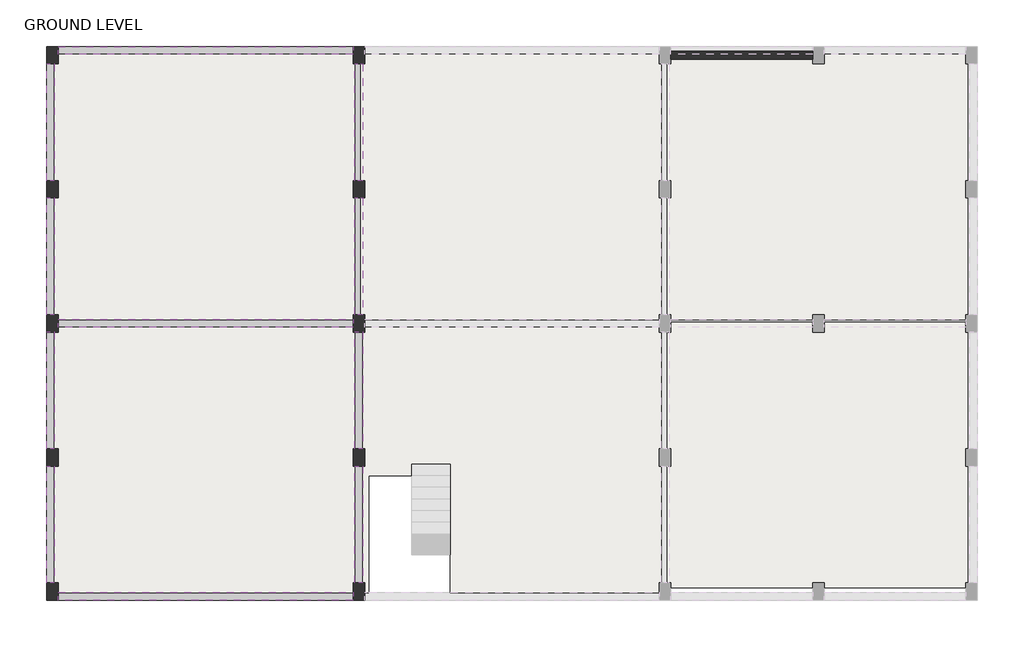
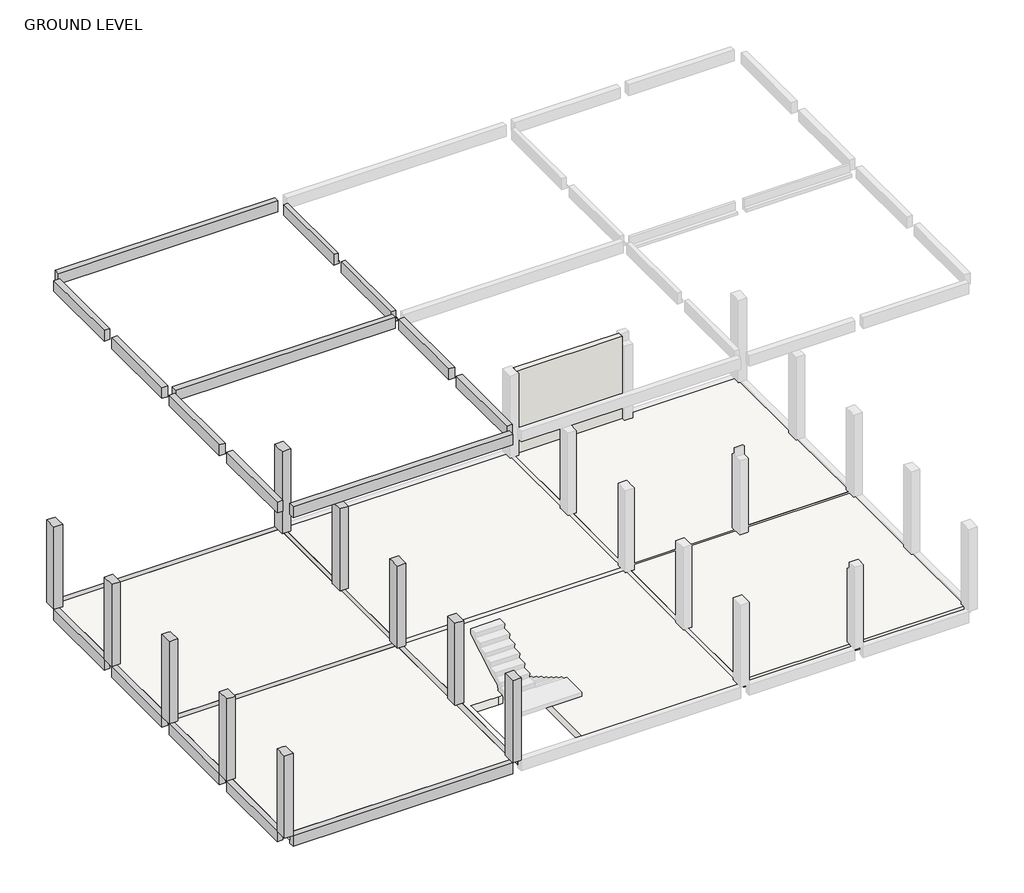
# One storey, part 1 of 2: 22 beams, 10 columns, 1 slab, 1 wall.
"""IFC4 building model written with IfcOpenShell, lengths in millimetres."""

from ifc_helpers import new_model, si_unit, frame, origin, place, context, project, spatial, polyline, outline, extrude, faceted_brep, element, save

model = new_model("IFC4")

# Units and contexts
model_context = context("Model", 3, world=origin())
ifc_project = project(units=[si_unit("LENGTHUNIT", "METRE", prefix="MILLI")], contexts=[model_context])

# Site, building, storey
site = spatial("IfcSite", under=ifc_project)
building = spatial("IfcBuilding", under=site)
storey = spatial("IfcBuildingStorey", under=building, Name="GROUND LEVEL", Elevation=0.0)

# Beams
placement = place(None, origin())
element("IfcBeam", 1, ObjectType="M_Concrete-Rectangular Beam : 200MMX400MM", at=placement, inside=storey, context=model_context, shape_type="Brep", body=[
    faceted_brep([(-3980.6874017, 15797.7008557, 0.0), (-3980.6874017, 15997.7008557, 0.0), (-11680.6874017, 15997.7008557, 0.0), (-11680.6874017, 15797.7008557, 0.0), (-3980.6874017, 15797.7008557, -400.0), (-3980.6874017, 15797.7008557, -300.0), (-11680.6874017, 15797.7008557, -300.0), (-11680.6874017, 15797.7008557, -400.0), (-3980.6874017, 15997.7008557, -400.0), (-11680.6874017, 15997.7008557, -400.0)], [[[0, 1, 2, 3]], [[4, 5, 0, 3, 6, 7]], [[8, 4, 7, 9]], [[1, 8, 9, 2]], [[2, 9, 7, 6, 3]], [[1, 0, 5, 4, 8]]]),
])
element("IfcBeam", 2, ObjectType="M_Concrete-Rectangular Beam : 200MMX400MM", at=placement, inside=storey, context=model_context, shape_type="Brep", body=[
    faceted_brep([(-11680.6874017, 1747.7008557, 0.0), (-11680.6874017, 1547.7008557, 0.0), (-3980.6874017, 1547.7008557, 0.0), (-3980.6874017, 1747.7008557, 0.0), (-11680.6874017, 1747.7008557, -400.0), (-11680.6874017, 1747.7008557, -300.0), (-3980.6874017, 1747.7008557, -300.0), (-3980.6874017, 1747.7008557, -400.0), (-11680.6874017, 1547.7008557, -400.0), (-3980.6874017, 1547.7008557, -400.0)], [[[0, 1, 2, 3]], [[4, 5, 0, 3, 6, 7]], [[8, 4, 7, 9]], [[1, 8, 9, 2]], [[1, 0, 5, 4, 8]], [[2, 9, 7, 6, 3]]]),
])
element("IfcBeam", 3, ObjectType="M_Concrete-Rectangular Beam : 200MMX400MM", at=placement, inside=storey, context=model_context, shape_type="Brep", body=[
    faceted_brep([(-3980.6874017, 8872.7008557, 0.0), (-11680.6874017, 8872.7008557, 0.0), (-11680.6874017, 8672.7008557, 0.0), (-3980.6874017, 8672.7008557, 0.0), (-11680.6874017, 8672.7008557, -300.0), (-11680.6874017, 8672.7008557, -400.0), (-3980.6874017, 8672.7008557, -400.0), (-3980.6874017, 8672.7008557, -300.0), (-11680.6874017, 8872.7008557, -400.0), (-3980.6874017, 8872.7008557, -400.0), (-3980.6874017, 8872.7008557, -300.0), (-11680.6874017, 8872.7008557, -300.0)], [[[0, 1, 2, 3]], [[3, 2, 4, 5, 6, 7]], [[6, 5, 8, 9]], [[1, 0, 10, 9, 8, 11]], [[8, 5, 4, 2, 1, 11]], [[0, 3, 7, 6, 9, 10]]]),
])
element("IfcBeam", 4, ObjectType="M_Concrete-Rectangular Beam : 200MMX400MM", at=placement, inside=storey, context=model_context, shape_type="Brep", body=[
    faceted_brep([(-11980.6874017, 12497.7008557, 0.0), (-11780.6874017, 12497.7008557, 0.0), (-11780.6874017, 15547.7008557, 0.0), (-11980.6874017, 15547.7008557, 0.0), (-11980.6874017, 12497.7008557, -400.0), (-11980.6874017, 15547.7008557, -400.0), (-11780.6874017, 12497.7008557, -400.0), (-11780.6874017, 15547.7008557, -400.0), (-11780.6874017, 12497.7008557, -300.0), (-11780.6874017, 15547.7008557, -300.0)], [[[0, 1, 2, 3]], [[4, 0, 3, 5]], [[6, 4, 5, 7]], [[1, 8, 6, 7, 9, 2]], [[2, 9, 7, 5, 3]], [[1, 0, 4, 6, 8]]]),
])
element("IfcBeam", 5, ObjectType="M_Concrete-Rectangular Beam : 200MMX400MM", at=placement, inside=storey, context=model_context, shape_type="Brep", body=[
    faceted_brep([(-11980.6874017, 8997.7008557, 0.0), (-11780.6874017, 8997.7008557, 0.0), (-11780.6874017, 12047.7008557, 0.0), (-11980.6874017, 12047.7008557, 0.0), (-11980.6874017, 8997.7008557, -400.0), (-11980.6874017, 12047.7008557, -400.0), (-11780.6874017, 8997.7008557, -400.0), (-11780.6874017, 12047.7008557, -400.0), (-11780.6874017, 8997.7008557, -300.0), (-11780.6874017, 12047.7008557, -300.0)], [[[0, 1, 2, 3]], [[4, 0, 3, 5]], [[6, 4, 5, 7]], [[1, 8, 6, 7, 9, 2]], [[1, 0, 4, 6, 8]], [[2, 9, 7, 5, 3]]]),
])
element("IfcBeam", 6, ObjectType="M_Concrete-Rectangular Beam : 200MMX400MM", at=placement, inside=storey, context=model_context, shape_type="Brep", body=[
    faceted_brep([(-11980.6874017, 5497.7008557, 0.0), (-11780.6874017, 5497.7008557, 0.0), (-11780.6874017, 8547.7008557, 0.0), (-11980.6874017, 8547.7008557, 0.0), (-11980.6874017, 5497.7008557, -400.0), (-11980.6874017, 8547.7008557, -400.0), (-11780.6874017, 5497.7008557, -400.0), (-11780.6874017, 8547.7008557, -400.0), (-11780.6874017, 5497.7008557, -300.0), (-11780.6874017, 8547.7008557, -300.0)], [[[0, 1, 2, 3]], [[4, 0, 3, 5]], [[6, 4, 5, 7]], [[1, 8, 6, 7, 9, 2]], [[2, 9, 7, 5, 3]], [[1, 0, 4, 6, 8]]]),
])
element("IfcBeam", 7, ObjectType="M_Concrete-Rectangular Beam : 200MMX400MM", at=placement, inside=storey, context=model_context, shape_type="Brep", body=[
    faceted_brep([(-11980.6874017, 1997.7008557, 0.0), (-11780.6874017, 1997.7008557, 0.0), (-11780.6874017, 5047.7008557, 0.0), (-11980.6874017, 5047.7008557, 0.0), (-11980.6874017, 1997.7008557, -400.0), (-11980.6874017, 5047.7008557, -400.0), (-11780.6874017, 1997.7008557, -400.0), (-11780.6874017, 5047.7008557, -400.0), (-11780.6874017, 1997.7008557, -300.0), (-11780.6874017, 5047.7008557, -300.0)], [[[0, 1, 2, 3]], [[4, 0, 3, 5]], [[6, 4, 5, 7]], [[1, 8, 6, 7, 9, 2]], [[1, 0, 4, 6, 8]], [[2, 9, 7, 5, 3]]]),
])
element("IfcBeam", 8, ObjectType="M_Concrete-Rectangular Beam : 200MMX400MM", at=placement, inside=storey, context=model_context, shape_type="Brep", body=[
    faceted_brep([(-3930.6874017, 5047.7008557, 0.0), (-3930.6874017, 1997.7008557, 0.0), (-3730.6874017, 1997.7008557, 0.0), (-3730.6874017, 5047.7008557, 0.0), (-3730.6874017, 1997.7008557, -300.0), (-3730.6874017, 1997.7008557, -400.0), (-3730.6874017, 5047.7008557, -400.0), (-3730.6874017, 5047.7008557, -300.0), (-3930.6874017, 1997.7008557, -400.0), (-3930.6874017, 5047.7008557, -400.0), (-3930.6874017, 5047.7008557, -300.0), (-3930.6874017, 1997.7008557, -300.0)], [[[0, 1, 2, 3]], [[3, 2, 4, 5, 6, 7]], [[6, 5, 8, 9]], [[1, 0, 10, 9, 8, 11]], [[8, 5, 4, 2, 1, 11]], [[0, 3, 7, 6, 9, 10]]]),
])
element("IfcBeam", 9, ObjectType="M_Concrete-Rectangular Beam : 200MMX400MM", at=placement, inside=storey, context=model_context, shape_type="Brep", body=[
    faceted_brep([(-3930.6874017, 8547.7008557, 0.0), (-3930.6874017, 5497.7008557, 0.0), (-3730.6874017, 5497.7008557, 0.0), (-3730.6874017, 8547.7008557, 0.0), (-3730.6874017, 5497.7008557, -300.0), (-3730.6874017, 5497.7008557, -400.0), (-3730.6874017, 8547.7008557, -400.0), (-3730.6874017, 8547.7008557, -300.0), (-3930.6874017, 5497.7008557, -400.0), (-3930.6874017, 8547.7008557, -400.0), (-3930.6874017, 8547.7008557, -300.0), (-3930.6874017, 5497.7008557, -300.0)], [[[0, 1, 2, 3]], [[3, 2, 4, 5, 6, 7]], [[6, 5, 8, 9]], [[1, 0, 10, 9, 8, 11]], [[0, 3, 7, 6, 9, 10]], [[8, 5, 4, 2, 1, 11]]]),
])
element("IfcBeam", 10, ObjectType="M_Concrete-Rectangular Beam : 200MMX400MM", at=placement, inside=storey, context=model_context, shape_type="Brep", body=[
    faceted_brep([(-3930.6874017, 12047.7008557, 0.0), (-3930.6874017, 8997.7008557, 0.0), (-3780.6874017, 8997.7008557, 0.0), (-3780.6874017, 12047.7008557, 0.0), (-3730.6874017, 8997.7008557, -400.0), (-3730.6874017, 12047.7008557, -400.0), (-3730.6874017, 12047.7008557, -300.0), (-3730.6874017, 8997.7008557, -300.0), (-3930.6874017, 8997.7008557, -400.0), (-3930.6874017, 12047.7008557, -400.0), (-3930.6874017, 12047.7008557, -300.0), (-3930.6874017, 8997.7008557, -300.0), (-3780.6874017, 12047.7008557, -300.0), (-3780.6874017, 8997.7008557, -300.0)], [[[0, 1, 2, 3]], [[4, 5, 6, 7]], [[5, 4, 8, 9]], [[1, 0, 10, 9, 8, 11]], [[5, 9, 10, 0, 3, 12, 6]], [[8, 4, 7, 13, 2, 1, 11]], [[12, 13, 7, 6]], [[13, 12, 3, 2]]]),
])
element("IfcBeam", 11, ObjectType="M_Concrete-Rectangular Beam : 200MMX400MM", at=placement, inside=storey, context=model_context, shape_type="Brep", body=[
    faceted_brep([(-3930.6874017, 15547.7008557, 0.0), (-3930.6874017, 12497.7008557, 0.0), (-3780.6874017, 12497.7008557, 0.0), (-3780.6874017, 15547.7008557, 0.0), (-3730.6874017, 12497.7008557, -400.0), (-3730.6874017, 15547.7008557, -400.0), (-3730.6874017, 15547.7008557, -300.0), (-3730.6874017, 12497.7008557, -300.0), (-3930.6874017, 12497.7008557, -400.0), (-3930.6874017, 15547.7008557, -400.0), (-3930.6874017, 15547.7008557, -300.0), (-3930.6874017, 12497.7008557, -300.0), (-3780.6874017, 15547.7008557, -300.0), (-3780.6874017, 12497.7008557, -300.0)], [[[0, 1, 2, 3]], [[4, 5, 6, 7]], [[5, 4, 8, 9]], [[1, 0, 10, 9, 8, 11]], [[5, 9, 10, 0, 3, 12, 6]], [[8, 4, 7, 13, 2, 1, 11]], [[12, 13, 7, 6]], [[13, 12, 3, 2]]]),
])
element("IfcBeam", 12, ObjectType="M_Concrete-Rectangular Beam : 200MMX400MM", at=placement, inside=storey, context=model_context, shape_type="Brep", body=[
    faceted_brep([(-3980.6874017, 15797.7008557, 12192.0), (-3980.6874017, 15997.7008557, 12192.0), (-11680.6874017, 15997.7008557, 12192.0), (-11680.6874017, 15797.7008557, 12192.0), (-3980.6874017, 15797.7008557, 11792.0), (-3980.6874017, 15797.7008557, 11892.0), (-11680.6874017, 15797.7008557, 11892.0), (-11680.6874017, 15797.7008557, 11792.0), (-3980.6874017, 15997.7008557, 11792.0), (-11680.6874017, 15997.7008557, 11792.0)], [[[0, 1, 2, 3]], [[4, 5, 0, 3, 6, 7]], [[8, 4, 7, 9]], [[1, 8, 9, 2]], [[2, 9, 7, 6, 3]], [[1, 0, 5, 4, 8]]]),
])
element("IfcBeam", 13, ObjectType="M_Concrete-Rectangular Beam : 200MMX400MM", at=placement, inside=storey, context=model_context, shape_type="Brep", body=[
    faceted_brep([(-11680.6874017, 1747.7008557, 12192.0), (-11680.6874017, 1547.7008557, 12192.0), (-3980.6874017, 1547.7008557, 12192.0), (-3980.6874017, 1747.7008557, 12192.0), (-11680.6874017, 1747.7008557, 11792.0), (-11680.6874017, 1747.7008557, 11892.0), (-3980.6874017, 1747.7008557, 11892.0), (-3980.6874017, 1747.7008557, 11792.0), (-11680.6874017, 1547.7008557, 11792.0), (-3980.6874017, 1547.7008557, 11792.0)], [[[0, 1, 2, 3]], [[4, 5, 0, 3, 6, 7]], [[8, 4, 7, 9]], [[1, 8, 9, 2]], [[1, 0, 5, 4, 8]], [[2, 9, 7, 6, 3]]]),
])
element("IfcBeam", 14, ObjectType="M_Concrete-Rectangular Beam : 200MMX400MM", at=placement, inside=storey, context=model_context, shape_type="Brep", body=[
    faceted_brep([(-3980.6874017, 8872.7008557, 12192.0), (-11680.6874017, 8872.7008557, 12192.0), (-11680.6874017, 8672.7008557, 12192.0), (-3980.6874017, 8672.7008557, 12192.0), (-11680.6874017, 8672.7008557, 11892.0), (-11680.6874017, 8672.7008557, 11792.0), (-3980.6874017, 8672.7008557, 11792.0), (-3980.6874017, 8672.7008557, 11892.0), (-11680.6874017, 8872.7008557, 11792.0), (-3980.6874017, 8872.7008557, 11792.0), (-3980.6874017, 8872.7008557, 11892.0), (-11680.6874017, 8872.7008557, 11892.0)], [[[0, 1, 2, 3]], [[3, 2, 4, 5, 6, 7]], [[6, 5, 8, 9]], [[1, 0, 10, 9, 8, 11]], [[8, 5, 4, 2, 1, 11]], [[0, 3, 7, 6, 9, 10]]]),
])
element("IfcBeam", 15, ObjectType="M_Concrete-Rectangular Beam : 200MMX400MM", at=placement, inside=storey, context=model_context, shape_type="Brep", body=[
    faceted_brep([(-11980.6874017, 12497.7008557, 12192.0), (-11780.6874017, 12497.7008557, 12192.0), (-11780.6874017, 15547.7008557, 12192.0), (-11980.6874017, 15547.7008557, 12192.0), (-11980.6874017, 12497.7008557, 11792.0), (-11980.6874017, 15547.7008557, 11792.0), (-11780.6874017, 12497.7008557, 11792.0), (-11780.6874017, 15547.7008557, 11792.0), (-11780.6874017, 12497.7008557, 11892.0), (-11780.6874017, 15547.7008557, 11892.0)], [[[0, 1, 2, 3]], [[4, 0, 3, 5]], [[6, 4, 5, 7]], [[1, 8, 6, 7, 9, 2]], [[2, 9, 7, 5, 3]], [[1, 0, 4, 6, 8]]]),
])
element("IfcBeam", 16, ObjectType="M_Concrete-Rectangular Beam : 200MMX400MM", at=placement, inside=storey, context=model_context, shape_type="Brep", body=[
    faceted_brep([(-11980.6874017, 8997.7008557, 12192.0), (-11780.6874017, 8997.7008557, 12192.0), (-11780.6874017, 12047.7008557, 12192.0), (-11980.6874017, 12047.7008557, 12192.0), (-11980.6874017, 8997.7008557, 11792.0), (-11980.6874017, 12047.7008557, 11792.0), (-11780.6874017, 8997.7008557, 11792.0), (-11780.6874017, 12047.7008557, 11792.0), (-11780.6874017, 8997.7008557, 11892.0), (-11780.6874017, 12047.7008557, 11892.0)], [[[0, 1, 2, 3]], [[4, 0, 3, 5]], [[6, 4, 5, 7]], [[1, 8, 6, 7, 9, 2]], [[1, 0, 4, 6, 8]], [[2, 9, 7, 5, 3]]]),
])
element("IfcBeam", 17, ObjectType="M_Concrete-Rectangular Beam : 200MMX400MM", at=placement, inside=storey, context=model_context, shape_type="Brep", body=[
    faceted_brep([(-11980.6874017, 5497.7008557, 12192.0), (-11780.6874017, 5497.7008557, 12192.0), (-11780.6874017, 8547.7008557, 12192.0), (-11980.6874017, 8547.7008557, 12192.0), (-11980.6874017, 5497.7008557, 11792.0), (-11980.6874017, 8547.7008557, 11792.0), (-11780.6874017, 5497.7008557, 11792.0), (-11780.6874017, 8547.7008557, 11792.0), (-11780.6874017, 5497.7008557, 11892.0), (-11780.6874017, 8547.7008557, 11892.0)], [[[0, 1, 2, 3]], [[4, 0, 3, 5]], [[6, 4, 5, 7]], [[1, 8, 6, 7, 9, 2]], [[2, 9, 7, 5, 3]], [[1, 0, 4, 6, 8]]]),
])
element("IfcBeam", 18, ObjectType="M_Concrete-Rectangular Beam : 200MMX400MM", at=placement, inside=storey, context=model_context, shape_type="Brep", body=[
    faceted_brep([(-11980.6874017, 1997.7008557, 12192.0), (-11780.6874017, 1997.7008557, 12192.0), (-11780.6874017, 5047.7008557, 12192.0), (-11980.6874017, 5047.7008557, 12192.0), (-11980.6874017, 1997.7008557, 11792.0), (-11980.6874017, 5047.7008557, 11792.0), (-11780.6874017, 1997.7008557, 11792.0), (-11780.6874017, 5047.7008557, 11792.0), (-11780.6874017, 1997.7008557, 11892.0), (-11780.6874017, 5047.7008557, 11892.0)], [[[0, 1, 2, 3]], [[4, 0, 3, 5]], [[6, 4, 5, 7]], [[1, 8, 6, 7, 9, 2]], [[1, 0, 4, 6, 8]], [[2, 9, 7, 5, 3]]]),
])
element("IfcBeam", 19, ObjectType="M_Concrete-Rectangular Beam : 200MMX400MM", at=placement, inside=storey, context=model_context, shape_type="Brep", body=[
    faceted_brep([(-3930.6874017, 5047.7008557, 12192.0), (-3930.6874017, 1997.7008557, 12192.0), (-3730.6874017, 1997.7008557, 12192.0), (-3730.6874017, 5047.7008557, 12192.0), (-3730.6874017, 1997.7008557, 11892.0), (-3730.6874017, 1997.7008557, 11792.0), (-3730.6874017, 5047.7008557, 11792.0), (-3730.6874017, 5047.7008557, 11892.0), (-3930.6874017, 1997.7008557, 11792.0), (-3930.6874017, 5047.7008557, 11792.0), (-3930.6874017, 5047.7008557, 11892.0), (-3930.6874017, 1997.7008557, 11892.0)], [[[0, 1, 2, 3]], [[3, 2, 4, 5, 6, 7]], [[6, 5, 8, 9]], [[1, 0, 10, 9, 8, 11]], [[8, 5, 4, 2, 1, 11]], [[0, 3, 7, 6, 9, 10]]]),
])
element("IfcBeam", 20, ObjectType="M_Concrete-Rectangular Beam : 200MMX400MM", at=placement, inside=storey, context=model_context, shape_type="Brep", body=[
    faceted_brep([(-3930.6874017, 8547.7008557, 12192.0), (-3930.6874017, 5497.7008557, 12192.0), (-3730.6874017, 5497.7008557, 12192.0), (-3730.6874017, 8547.7008557, 12192.0), (-3730.6874017, 5497.7008557, 11892.0), (-3730.6874017, 5497.7008557, 11792.0), (-3730.6874017, 8547.7008557, 11792.0), (-3730.6874017, 8547.7008557, 11892.0), (-3930.6874017, 5497.7008557, 11792.0), (-3930.6874017, 8547.7008557, 11792.0), (-3930.6874017, 8547.7008557, 11892.0), (-3930.6874017, 5497.7008557, 11892.0)], [[[0, 1, 2, 3]], [[3, 2, 4, 5, 6, 7]], [[6, 5, 8, 9]], [[1, 0, 10, 9, 8, 11]], [[0, 3, 7, 6, 9, 10]], [[8, 5, 4, 2, 1, 11]]]),
])
element("IfcBeam", 21, ObjectType="M_Concrete-Rectangular Beam : 200MMX400MM", at=placement, inside=storey, context=model_context, shape_type="Brep", body=[
    faceted_brep([(-3930.6874017, 12047.7008557, 12192.0), (-3930.6874017, 8997.7008557, 12192.0), (-3780.6874017, 8997.7008557, 12192.0), (-3780.6874017, 12047.7008557, 12192.0), (-3730.6874017, 8997.7008557, 11792.0), (-3730.6874017, 12047.7008557, 11792.0), (-3730.6874017, 12047.7008557, 11892.0), (-3730.6874017, 8997.7008557, 11892.0), (-3930.6874017, 8997.7008557, 11792.0), (-3930.6874017, 12047.7008557, 11792.0), (-3930.6874017, 12047.7008557, 11892.0), (-3930.6874017, 8997.7008557, 11892.0), (-3780.6874017, 12047.7008557, 11892.0), (-3780.6874017, 8997.7008557, 11892.0)], [[[0, 1, 2, 3]], [[4, 5, 6, 7]], [[5, 4, 8, 9]], [[1, 0, 10, 9, 8, 11]], [[5, 9, 10, 0, 3, 12, 6]], [[8, 4, 7, 13, 2, 1, 11]], [[12, 13, 7, 6]], [[13, 12, 3, 2]]]),
])
element("IfcBeam", 22, ObjectType="M_Concrete-Rectangular Beam : 200MMX400MM", at=placement, inside=storey, context=model_context, shape_type="Brep", body=[
    faceted_brep([(-3930.6874017, 15547.7008557, 12192.0), (-3930.6874017, 12497.7008557, 12192.0), (-3780.6874017, 12497.7008557, 12192.0), (-3780.6874017, 15547.7008557, 12192.0), (-3730.6874017, 12497.7008557, 11792.0), (-3730.6874017, 15547.7008557, 11792.0), (-3730.6874017, 15547.7008557, 11892.0), (-3730.6874017, 12497.7008557, 11892.0), (-3930.6874017, 12497.7008557, 11792.0), (-3930.6874017, 15547.7008557, 11792.0), (-3930.6874017, 15547.7008557, 11892.0), (-3930.6874017, 12497.7008557, 11892.0), (-3780.6874017, 15547.7008557, 11892.0), (-3780.6874017, 12497.7008557, 11892.0)], [[[0, 1, 2, 3]], [[4, 5, 6, 7]], [[5, 4, 8, 9]], [[1, 0, 10, 9, 8, 11]], [[5, 9, 10, 0, 3, 12, 6]], [[8, 4, 7, 13, 2, 1, 11]], [[12, 13, 7, 6]], [[13, 12, 3, 2]]]),
])

# Columns
element("IfcColumn", 23, ObjectType="M_Concrete-Rectangular-Column : 300 x 450mm", at=placement, inside=storey, context=model_context, shape_type="Brep", body=[
    faceted_brep([(-11680.6874017, 15997.7008557, 0.0), (-11680.6874017, 15547.7008557, 0.0), (-11980.6874017, 15547.7008557, 0.0), (-11980.6874017, 15997.7008557, 0.0), (-11680.6874017, 15997.7008557, 3048.0), (-11680.6874017, 15797.7008557, 3048.0), (-11680.6874017, 15547.7008557, 3048.0), (-11680.6874017, 15547.7008557, 2748.0), (-11780.6874017, 15547.7008557, 3048.0), (-11980.6874017, 15547.7008557, 3048.0), (-11980.6874017, 15997.7008557, 3048.0)], [[[0, 1, 2, 3]], [[1, 0, 4, 5, 6, 7]], [[2, 1, 7, 6, 8, 9]], [[3, 2, 9, 10]], [[0, 3, 10, 4]], [[10, 9, 8, 6, 5, 4]]]),
])
element("IfcColumn", 24, ObjectType="M_Concrete-Rectangular-Column : 300 x 450mm", at=placement, inside=storey, context=model_context, shape_type="Brep", body=[
    faceted_brep([(-11680.6874017, 8997.7008557, 0.0), (-11680.6874017, 8547.7008557, 0.0), (-11980.6874017, 8547.7008557, 0.0), (-11980.6874017, 8997.7008557, 0.0), (-11680.6874017, 8997.7008557, 2748.0), (-11680.6874017, 8997.7008557, 3048.0), (-11680.6874017, 8872.7008557, 3048.0), (-11680.6874017, 8672.7008557, 3048.0), (-11680.6874017, 8547.7008557, 3048.0), (-11680.6874017, 8547.7008557, 2748.0), (-11780.6874017, 8547.7008557, 3048.0), (-11980.6874017, 8547.7008557, 3048.0), (-11980.6874017, 8997.7008557, 3048.0), (-11780.6874017, 8997.7008557, 3048.0)], [[[0, 1, 2, 3]], [[1, 0, 4, 5, 6, 7, 8, 9]], [[2, 1, 9, 8, 10, 11]], [[3, 2, 11, 12]], [[0, 3, 12, 13, 5, 4]], [[12, 11, 10, 8, 7, 6, 5, 13]]]),
])
element("IfcColumn", 25, ObjectType="M_Concrete-Rectangular-Column : 300 x 450mm", at=placement, inside=storey, context=model_context, shape_type="Brep", body=[
    faceted_brep([(-11680.6874017, 1997.7008557, 0.0), (-11680.6874017, 1547.7008557, 0.0), (-11980.6874017, 1547.7008557, 0.0), (-11980.6874017, 1997.7008557, 0.0), (-11680.6874017, 1997.7008557, 2748.0), (-11680.6874017, 1997.7008557, 3048.0), (-11680.6874017, 1747.7008557, 3048.0), (-11680.6874017, 1547.7008557, 3048.0), (-11980.6874017, 1547.7008557, 3048.0), (-11980.6874017, 1997.7008557, 3048.0), (-11780.6874017, 1997.7008557, 3048.0)], [[[0, 1, 2, 3]], [[1, 0, 4, 5, 6, 7]], [[2, 1, 7, 8]], [[3, 2, 8, 9]], [[0, 3, 9, 10, 5, 4]], [[8, 7, 6, 5, 10, 9]]]),
])
element("IfcColumn", 26, ObjectType="M_Concrete-Rectangular-Column : 300 x 450mm", at=placement, inside=storey, context=model_context, shape_type="Brep", body=[
    faceted_brep([(-3680.6874017, 15997.7008557, 0.0), (-3680.6874017, 15547.7008557, 0.0), (-3980.6874017, 15547.7008557, 0.0), (-3980.6874017, 15997.7008557, 0.0), (-3680.6874017, 15997.7008557, 3048.0), (-3680.6874017, 15797.7008557, 3048.0), (-3680.6874017, 15547.7008557, 3048.0), (-3680.6874017, 15547.7008557, 2748.0), (-3780.6874017, 15547.7008557, 3048.0), (-3930.6874017, 15547.7008557, 3048.0), (-3980.6874017, 15547.7008557, 3048.0), (-3980.6874017, 15547.7008557, 2748.0), (-3980.6874017, 15797.7008557, 3048.0), (-3980.6874017, 15997.7008557, 3048.0)], [[[0, 1, 2, 3]], [[1, 0, 4, 5, 6, 7]], [[2, 1, 7, 6, 8, 9, 10, 11]], [[3, 2, 11, 10, 12, 13]], [[0, 3, 13, 4]], [[4, 13, 12, 10, 9, 8, 6, 5]]]),
])
element("IfcColumn", 27, ObjectType="M_Concrete-Rectangular-Column : 300 x 450mm", at=placement, inside=storey, context=model_context, shape_type="Brep", body=[
    faceted_brep([(-3680.6874017, 12497.7008557, 0.0), (-3680.6874017, 12047.7008557, 0.0), (-3980.6874017, 12047.7008557, 0.0), (-3980.6874017, 12497.7008557, 0.0), (-3680.6874017, 12497.7008557, 2748.0), (-3680.6874017, 12497.7008557, 3048.0), (-3680.6874017, 12047.7008557, 3048.0), (-3680.6874017, 12047.7008557, 2748.0), (-3780.6874017, 12047.7008557, 3048.0), (-3930.6874017, 12047.7008557, 3048.0), (-3980.6874017, 12047.7008557, 3048.0), (-3980.6874017, 12047.7008557, 2748.0), (-3980.6874017, 12497.7008557, 3048.0), (-3980.6874017, 12497.7008557, 2748.0), (-3930.6874017, 12497.7008557, 3048.0), (-3780.6874017, 12497.7008557, 3048.0)], [[[0, 1, 2, 3]], [[1, 0, 4, 5, 6, 7]], [[2, 1, 7, 6, 8, 9, 10, 11]], [[3, 2, 11, 10, 12, 13]], [[0, 3, 13, 12, 14, 15, 5, 4]], [[6, 5, 15, 14, 12, 10, 9, 8]]]),
])
element("IfcColumn", 28, ObjectType="M_Concrete-Rectangular-Column : 300 x 450mm", at=placement, inside=storey, context=model_context, shape_type="Brep", body=[
    faceted_brep([(-3680.6874017, 8997.7008557, 0.0), (-3680.6874017, 8547.7008557, 0.0), (-3980.6874017, 8547.7008557, 0.0), (-3980.6874017, 8997.7008557, 0.0), (-3680.6874017, 8997.7008557, 2748.0), (-3680.6874017, 8997.7008557, 3048.0), (-3680.6874017, 8872.7008557, 3048.0), (-3680.6874017, 8672.7008557, 3048.0), (-3680.6874017, 8547.7008557, 3048.0), (-3680.6874017, 8547.7008557, 2748.0), (-3730.6874017, 8547.7008557, 3048.0), (-3930.6874017, 8547.7008557, 3048.0), (-3980.6874017, 8547.7008557, 3048.0), (-3980.6874017, 8547.7008557, 2748.0), (-3980.6874017, 8672.7008557, 3048.0), (-3980.6874017, 8872.7008557, 3048.0), (-3980.6874017, 8997.7008557, 3048.0), (-3980.6874017, 8997.7008557, 2748.0), (-3930.6874017, 8997.7008557, 3048.0), (-3780.6874017, 8997.7008557, 3048.0)], [[[0, 1, 2, 3]], [[1, 0, 4, 5, 6, 7, 8, 9]], [[2, 1, 9, 8, 10, 11, 12, 13]], [[3, 2, 13, 12, 14, 15, 16, 17]], [[0, 3, 17, 16, 18, 19, 5, 4]], [[18, 16, 15, 14, 12, 11, 10, 8, 7, 6, 5, 19]]]),
])
element("IfcColumn", 29, ObjectType="M_Concrete-Rectangular-Column : 300 x 450mm", at=placement, inside=storey, context=model_context, shape_type="Brep", body=[
    faceted_brep([(-3680.6874017, 5497.7008557, 0.0), (-3680.6874017, 5047.7008557, 0.0), (-3980.6874017, 5047.7008557, 0.0), (-3980.6874017, 5497.7008557, 0.0), (-3680.6874017, 5497.7008557, 2748.0), (-3680.6874017, 5497.7008557, 3048.0), (-3680.6874017, 5047.7008557, 3048.0), (-3680.6874017, 5047.7008557, 2748.0), (-3730.6874017, 5047.7008557, 3048.0), (-3930.6874017, 5047.7008557, 3048.0), (-3980.6874017, 5047.7008557, 3048.0), (-3980.6874017, 5047.7008557, 2748.0), (-3980.6874017, 5497.7008557, 3048.0), (-3980.6874017, 5497.7008557, 2748.0), (-3930.6874017, 5497.7008557, 3048.0), (-3730.6874017, 5497.7008557, 3048.0)], [[[0, 1, 2, 3]], [[1, 0, 4, 5, 6, 7]], [[2, 1, 7, 6, 8, 9, 10, 11]], [[3, 2, 11, 10, 12, 13]], [[0, 3, 13, 12, 14, 15, 5, 4]], [[6, 5, 15, 14, 12, 10, 9, 8]]]),
])
element("IfcColumn", 30, ObjectType="M_Concrete-Rectangular-Column : 300 x 450mm", at=placement, inside=storey, context=model_context, shape_type="Brep", body=[
    faceted_brep([(-3680.6874017, 1997.7008557, 0.0), (-3680.6874017, 1547.7008557, 0.0), (-3980.6874017, 1547.7008557, 0.0), (-3980.6874017, 1997.7008557, 0.0), (-3680.6874017, 1997.7008557, 2748.0), (-3680.6874017, 1997.7008557, 3048.0), (-3680.6874017, 1747.7008557, 3048.0), (-3680.6874017, 1547.7008557, 3048.0), (-3980.6874017, 1547.7008557, 3048.0), (-3980.6874017, 1747.7008557, 3048.0), (-3980.6874017, 1997.7008557, 3048.0), (-3980.6874017, 1997.7008557, 2748.0), (-3930.6874017, 1997.7008557, 3048.0), (-3730.6874017, 1997.7008557, 3048.0)], [[[0, 1, 2, 3]], [[1, 0, 4, 5, 6, 7]], [[2, 1, 7, 8]], [[3, 2, 8, 9, 10, 11]], [[0, 3, 11, 10, 12, 13, 5, 4]], [[8, 7, 6, 5, 13, 12, 10, 9]]]),
])
element("IfcColumn", 31, ObjectType="M_Concrete-Rectangular-Column : 300 x 450mm", at=placement, inside=storey, context=model_context, shape_type="Brep", body=[
    faceted_brep([(-11680.6874017, 12497.7008557, 0.0), (-11680.6874017, 12047.7008557, 0.0), (-11980.6874017, 12047.7008557, 0.0), (-11980.6874017, 12497.7008557, 0.0), (-11680.6874017, 12497.7008557, 2748.0), (-11680.6874017, 12497.7008557, 3048.0), (-11680.6874017, 12047.7008557, 3048.0), (-11680.6874017, 12047.7008557, 2748.0), (-11780.6874017, 12047.7008557, 3048.0), (-11980.6874017, 12047.7008557, 3048.0), (-11980.6874017, 12497.7008557, 3048.0), (-11780.6874017, 12497.7008557, 3048.0)], [[[0, 1, 2, 3]], [[1, 0, 4, 5, 6, 7]], [[2, 1, 7, 6, 8, 9]], [[3, 2, 9, 10]], [[0, 3, 10, 11, 5, 4]], [[6, 5, 11, 10, 9, 8]]]),
])
element("IfcColumn", 32, ObjectType="M_Concrete-Rectangular-Column : 300 x 450mm", at=placement, inside=storey, context=model_context, shape_type="Brep", body=[
    faceted_brep([(-11680.6874017, 5497.7008557, 0.0), (-11680.6874017, 5047.7008557, 0.0), (-11980.6874017, 5047.7008557, 0.0), (-11980.6874017, 5497.7008557, 0.0), (-11680.6874017, 5497.7008557, 2748.0), (-11680.6874017, 5497.7008557, 3048.0), (-11680.6874017, 5047.7008557, 3048.0), (-11680.6874017, 5047.7008557, 2748.0), (-11780.6874017, 5047.7008557, 3048.0), (-11980.6874017, 5047.7008557, 3048.0), (-11980.6874017, 5497.7008557, 3048.0), (-11780.6874017, 5497.7008557, 3048.0)], [[[0, 1, 2, 3]], [[1, 0, 4, 5, 6, 7]], [[2, 1, 7, 6, 8, 9]], [[3, 2, 9, 10]], [[0, 3, 10, 11, 5, 4]], [[6, 5, 11, 10, 9, 8]]]),
])

# Slab
element("IfcSlab", 33, ObjectType="Generic 300mm", at=placement, inside=storey, context=model_context, shape_type="Brep", body=[
    faceted_brep([(-11680.6874017, 15547.7008557, -300.0), (-11680.6874017, 15797.7008557, -300.0), (-3980.6874017, 15797.7008557, -300.0), (-3980.6874017, 15547.7008557, -300.0), (-3930.6874017, 15547.7008557, -300.0), (-3930.6874017, 12497.7008557, -300.0), (-3980.6874017, 12497.7008557, -300.0), (-3980.6874017, 12047.7008557, -300.0), (-3930.6874017, 12047.7008557, -300.0), (-3930.6874017, 8997.7008557, -300.0), (-3980.6874017, 8997.7008557, -300.0), (-3980.6874017, 8872.7008557, -300.0), (-11680.6874017, 8872.7008557, -300.0), (-11680.6874017, 8997.7008557, -300.0), (-11780.6874017, 8997.7008557, -300.0), (-11780.6874017, 12047.7008557, -300.0), (-11680.6874017, 12047.7008557, -300.0), (-11680.6874017, 12497.7008557, -300.0), (-11780.6874017, 12497.7008557, -300.0), (-11780.6874017, 15547.7008557, -300.0), (-11680.6874017, 15797.7008557, 0.0), (-11680.6874017, 15547.7008557, 0.0), (-11780.6874017, 15547.7008557, 0.0), (-11780.6874017, 12497.7008557, 0.0), (-11680.6874017, 12497.7008557, 0.0), (-11680.6874017, 12047.7008557, 0.0), (-11780.6874017, 12047.7008557, 0.0), (-11780.6874017, 8997.7008557, 0.0), (-11680.6874017, 8997.7008557, 0.0), (-11680.6874017, 8872.7008557, 0.0), (-3980.6874017, 8872.7008557, 0.0), (-3980.6874017, 8997.7008557, 0.0), (-3930.6874017, 8997.7008557, 0.0), (-3930.6874017, 12047.7008557, 0.0), (-3980.6874017, 12047.7008557, 0.0), (-3980.6874017, 12497.7008557, 0.0), (-3930.6874017, 12497.7008557, 0.0), (-3930.6874017, 15547.7008557, 0.0), (-3980.6874017, 15547.7008557, 0.0), (-3980.6874017, 15797.7008557, 0.0)], [[[0, 1, 2, 3, 4, 5, 6, 7, 8, 9, 10, 11, 12, 13, 14, 15, 16, 17, 18, 19]], [[20, 21, 22, 23, 24, 25, 26, 27, 28, 29, 30, 31, 32, 33, 34, 35, 36, 37, 38, 39]], [[1, 0, 21, 20]], [[2, 1, 20, 39]], [[3, 2, 39, 38]], [[4, 3, 38, 37]], [[5, 4, 37, 36]], [[6, 5, 36, 35]], [[7, 6, 35, 34]], [[8, 7, 34, 33]], [[9, 8, 33, 32]], [[10, 9, 32, 31]], [[11, 10, 31, 30]], [[12, 11, 30, 29]], [[13, 12, 29, 28]], [[14, 13, 28, 27]], [[15, 14, 27, 26]], [[16, 15, 26, 25]], [[17, 16, 25, 24]], [[18, 17, 24, 23]], [[19, 18, 23, 22]], [[0, 19, 22, 21]]]),
    faceted_brep([(-3680.6874017, 15547.7008557, -300.0), (-3680.6874017, 15797.7008557, -300.0), (4019.3125983, 15797.7008557, -300.0), (4019.3125983, 15547.7008557, -300.0), (4069.3125983, 15547.7008557, -300.0), (4069.3125983, 12497.7008557, -300.0), (4019.3125983, 12497.7008557, -300.0), (4019.3125983, 12047.7008557, -300.0), (4069.3125983, 12047.7008557, -300.0), (4069.3125983, 8997.7008557, -300.0), (4019.3125983, 8997.7008557, -300.0), (4019.3125983, 8872.7008557, -300.0), (-3680.6874017, 8872.7008557, -300.0), (-3680.6874017, 8997.7008557, -300.0), (-3730.6874017, 8997.7008557, -300.0), (-3780.6874017, 8997.7008557, -300.0), (-3780.6874017, 12047.7008557, -300.0), (-3730.6874017, 12047.7008557, -300.0), (-3680.6874017, 12047.7008557, -300.0), (-3680.6874017, 12497.7008557, -300.0), (-3730.6874017, 12497.7008557, -300.0), (-3780.6874017, 12497.7008557, -300.0), (-3780.6874017, 15547.7008557, -300.0), (-3730.6874017, 15547.7008557, -300.0), (-3680.6874017, 15797.7008557, 0.0), (-3680.6874017, 15547.7008557, 0.0), (-3780.6874017, 15547.7008557, 0.0), (-3780.6874017, 12497.7008557, 0.0), (-3680.6874017, 12497.7008557, 0.0), (-3680.6874017, 12047.7008557, 0.0), (-3780.6874017, 12047.7008557, 0.0), (-3780.6874017, 8997.7008557, 0.0), (-3680.6874017, 8997.7008557, 0.0), (-3680.6874017, 8872.7008557, 0.0), (4019.3125983, 8872.7008557, 0.0), (4019.3125983, 8997.7008557, 0.0), (4069.3125983, 8997.7008557, 0.0), (4069.3125983, 12047.7008557, 0.0), (4019.3125983, 12047.7008557, 0.0), (4019.3125983, 12497.7008557, 0.0), (4069.3125983, 12497.7008557, 0.0), (4069.3125983, 15547.7008557, 0.0), (4019.3125983, 15547.7008557, 0.0), (4019.3125983, 15797.7008557, 0.0)], [[[0, 1, 2, 3, 4, 5, 6, 7, 8, 9, 10, 11, 12, 13, 14, 15, 16, 17, 18, 19, 20, 21, 22, 23]], [[24, 25, 26, 27, 28, 29, 30, 31, 32, 33, 34, 35, 36, 37, 38, 39, 40, 41, 42, 43]], [[1, 0, 25, 24]], [[2, 1, 24, 43]], [[3, 2, 43, 42]], [[4, 3, 42, 41]], [[5, 4, 41, 40]], [[6, 5, 40, 39]], [[7, 6, 39, 38]], [[8, 7, 38, 37]], [[9, 8, 37, 36]], [[10, 9, 36, 35]], [[11, 10, 35, 34]], [[12, 11, 34, 33]], [[13, 12, 33, 32]], [[15, 14, 13, 32, 31]], [[16, 15, 31, 30]], [[18, 17, 16, 30, 29]], [[19, 18, 29, 28]], [[21, 20, 19, 28, 27]], [[22, 21, 27, 26]], [[0, 23, 22, 26, 25]]]),
    faceted_brep([(4319.3125983, 15547.7008557, -300.0), (4319.3125983, 15797.7008557, -300.0), (8019.3125983, 15797.7008557, -300.0), (8319.3125983, 15797.7008557, -300.0), (12019.3125983, 15797.7008557, -300.0), (12019.3125983, 15547.7008557, -300.0), (12069.3125983, 15547.7008557, -300.0), (12069.3125983, 12497.7008557, -300.0), (12019.3125983, 12497.7008557, -300.0), (12019.3125983, 12047.7008557, -300.0), (12069.3125983, 12047.7008557, -300.0), (12069.3125983, 8997.7008557, -300.0), (12019.3125983, 8997.7008557, -300.0), (12019.3125983, 8872.7008557, -300.0), (8319.3125983, 8872.7008557, -300.0), (8019.3125983, 8872.7008557, -300.0), (4319.3125983, 8872.7008557, -300.0), (4319.3125983, 8997.7008557, -300.0), (4269.3125983, 8997.7008557, -300.0), (4219.3125983, 8997.7008557, -300.0), (4219.3125983, 12047.7008557, -300.0), (4269.3125983, 12047.7008557, -300.0), (4319.3125983, 12047.7008557, -300.0), (4319.3125983, 12497.7008557, -300.0), (4269.3125983, 12497.7008557, -300.0), (4219.3125983, 12497.7008557, -300.0), (4219.3125983, 15547.7008557, -300.0), (4269.3125983, 15547.7008557, -300.0), (4319.3125983, 15797.7008557, 0.0), (4319.3125983, 15547.7008557, 0.0), (4219.3125983, 15547.7008557, 0.0), (4219.3125983, 12497.7008557, 0.0), (4319.3125983, 12497.7008557, 0.0), (4319.3125983, 12047.7008557, 0.0), (4219.3125983, 12047.7008557, 0.0), (4219.3125983, 8997.7008557, 0.0), (4319.3125983, 8997.7008557, 0.0), (4319.3125983, 8872.7008557, 0.0), (8019.3125983, 8872.7008557, 0.0), (8319.3125983, 8872.7008557, 0.0), (12019.3125983, 8872.7008557, 0.0), (12019.3125983, 8997.7008557, 0.0), (12069.3125983, 8997.7008557, 0.0), (12069.3125983, 12047.7008557, 0.0), (12019.3125983, 12047.7008557, 0.0), (12019.3125983, 12497.7008557, 0.0), (12069.3125983, 12497.7008557, 0.0), (12069.3125983, 15547.7008557, 0.0), (12019.3125983, 15547.7008557, 0.0), (12019.3125983, 15797.7008557, 0.0), (8319.3125983, 15797.7008557, 0.0), (8019.3125983, 15797.7008557, 0.0)], [[[0, 1, 2, 3, 4, 5, 6, 7, 8, 9, 10, 11, 12, 13, 14, 15, 16, 17, 18, 19, 20, 21, 22, 23, 24, 25, 26, 27]], [[28, 29, 30, 31, 32, 33, 34, 35, 36, 37, 38, 39, 40, 41, 42, 43, 44, 45, 46, 47, 48, 49, 50, 51]], [[1, 0, 29, 28]], [[4, 3, 2, 1, 28, 51, 50, 49]], [[5, 4, 49, 48]], [[6, 5, 48, 47]], [[7, 6, 47, 46]], [[8, 7, 46, 45]], [[9, 8, 45, 44]], [[10, 9, 44, 43]], [[11, 10, 43, 42]], [[12, 11, 42, 41]], [[13, 12, 41, 40]], [[16, 15, 14, 13, 40, 39, 38, 37]], [[17, 16, 37, 36]], [[19, 18, 17, 36, 35]], [[20, 19, 35, 34]], [[22, 21, 20, 34, 33]], [[23, 22, 33, 32]], [[25, 24, 23, 32, 31]], [[26, 25, 31, 30]], [[0, 27, 26, 30, 29]]]),
    faceted_brep([(-3680.6874017, 8547.7008557, -300.0), (-3680.6874017, 8672.7008557, -300.0), (4019.3125983, 8672.7008557, -300.0), (4019.3125983, 8547.7008557, -300.0), (4069.3125983, 8547.7008557, -300.0), (4069.3125983, 5497.7008557, -300.0), (4019.3125983, 5497.7008557, -300.0), (4019.3125983, 5047.7008557, -300.0), (4069.3125983, 5047.7008557, -300.0), (4069.3125983, 1997.7008557, -300.0), (4019.3125983, 1997.7008557, -300.0), (4019.3125983, 1747.7008557, -300.0), (-1437.0874017, 1747.7008557, -300.0), (-1437.0874017, 5100.5008557, -300.0), (-2453.0874017, 5100.5008557, -300.0), (-2453.0874017, 4795.7008557, -300.0), (-2593.0874017, 4795.7008557, -300.0), (-3570.6874017, 4795.7008557, -300.0), (-3570.6874017, 1747.7008557, -300.0), (-3680.6874017, 1747.7008557, -300.0), (-3680.6874017, 1997.7008557, -300.0), (-3730.6874017, 1997.7008557, -300.0), (-3730.6874017, 5047.7008557, -300.0), (-3680.6874017, 5047.7008557, -300.0), (-3680.6874017, 5497.7008557, -300.0), (-3730.6874017, 5497.7008557, -300.0), (-3730.6874017, 8547.7008557, -300.0), (-3680.6874017, 8672.7008557, 0.0), (-3680.6874017, 8547.7008557, 0.0), (-3730.6874017, 8547.7008557, 0.0), (-3730.6874017, 5497.7008557, 0.0), (-3680.6874017, 5497.7008557, 0.0), (-3680.6874017, 5047.7008557, 0.0), (-3730.6874017, 5047.7008557, 0.0), (-3730.6874017, 1997.7008557, 0.0), (-3680.6874017, 1997.7008557, 0.0), (-3680.6874017, 1747.7008557, 0.0), (-3570.6874017, 1747.7008557, 0.0), (-3570.6874017, 4795.7008557, 0.0), (-2593.0874017, 4795.7008557, 0.0), (-2453.0874017, 4795.7008557, 0.0), (-2453.0874017, 5100.5008557, 0.0), (-1437.0874017, 5100.5008557, 0.0), (-1437.0874017, 1747.7008557, 0.0), (4019.3125983, 1747.7008557, 0.0), (4019.3125983, 1997.7008557, 0.0), (4069.3125983, 1997.7008557, 0.0), (4069.3125983, 5047.7008557, 0.0), (4019.3125983, 5047.7008557, 0.0), (4019.3125983, 5497.7008557, 0.0), (4069.3125983, 5497.7008557, 0.0), (4069.3125983, 8547.7008557, 0.0), (4019.3125983, 8547.7008557, 0.0), (4019.3125983, 8672.7008557, 0.0)], [[[0, 1, 2, 3, 4, 5, 6, 7, 8, 9, 10, 11, 12, 13, 14, 15, 16, 17, 18, 19, 20, 21, 22, 23, 24, 25, 26]], [[27, 28, 29, 30, 31, 32, 33, 34, 35, 36, 37, 38, 39, 40, 41, 42, 43, 44, 45, 46, 47, 48, 49, 50, 51, 52, 53]], [[1, 0, 28, 27]], [[2, 1, 27, 53]], [[3, 2, 53, 52]], [[4, 3, 52, 51]], [[5, 4, 51, 50]], [[6, 5, 50, 49]], [[7, 6, 49, 48]], [[8, 7, 48, 47]], [[9, 8, 47, 46]], [[10, 9, 46, 45]], [[11, 10, 45, 44]], [[11, 44, 43, 12]], [[36, 19, 18, 37]], [[20, 19, 36, 35]], [[21, 20, 35, 34]], [[22, 21, 34, 33]], [[23, 22, 33, 32]], [[24, 23, 32, 31]], [[25, 24, 31, 30]], [[26, 25, 30, 29]], [[0, 26, 29, 28]], [[42, 13, 12, 43]], [[13, 42, 41, 14]], [[14, 41, 40, 15]], [[15, 40, 39, 16]], [[16, 39, 38, 17]], [[17, 38, 37, 18]]]),
    faceted_brep([(-3980.6874017, 1747.7008557, -300.0), (-11680.6874017, 1747.7008557, -300.0), (-11680.6874017, 1997.7008557, -300.0), (-11780.6874017, 1997.7008557, -300.0), (-11780.6874017, 5047.7008557, -300.0), (-11680.6874017, 5047.7008557, -300.0), (-11680.6874017, 5497.7008557, -300.0), (-11780.6874017, 5497.7008557, -300.0), (-11780.6874017, 8547.7008557, -300.0), (-11680.6874017, 8547.7008557, -300.0), (-11680.6874017, 8672.7008557, -300.0), (-3980.6874017, 8672.7008557, -300.0), (-3980.6874017, 8547.7008557, -300.0), (-3930.6874017, 8547.7008557, -300.0), (-3930.6874017, 5497.7008557, -300.0), (-3980.6874017, 5497.7008557, -300.0), (-3980.6874017, 5047.7008557, -300.0), (-3930.6874017, 5047.7008557, -300.0), (-3930.6874017, 1997.7008557, -300.0), (-3980.6874017, 1997.7008557, -300.0), (-11680.6874017, 1747.7008557, 0.0), (-3980.6874017, 1747.7008557, 0.0), (-3980.6874017, 1997.7008557, 0.0), (-3930.6874017, 1997.7008557, 0.0), (-3930.6874017, 5047.7008557, 0.0), (-3980.6874017, 5047.7008557, 0.0), (-3980.6874017, 5497.7008557, 0.0), (-3930.6874017, 5497.7008557, 0.0), (-3930.6874017, 8547.7008557, 0.0), (-3980.6874017, 8547.7008557, 0.0), (-3980.6874017, 8672.7008557, 0.0), (-11680.6874017, 8672.7008557, 0.0), (-11680.6874017, 8547.7008557, 0.0), (-11780.6874017, 8547.7008557, 0.0), (-11780.6874017, 5497.7008557, 0.0), (-11680.6874017, 5497.7008557, 0.0), (-11680.6874017, 5047.7008557, 0.0), (-11780.6874017, 5047.7008557, 0.0), (-11780.6874017, 1997.7008557, 0.0), (-11680.6874017, 1997.7008557, 0.0)], [[[0, 1, 2, 3, 4, 5, 6, 7, 8, 9, 10, 11, 12, 13, 14, 15, 16, 17, 18, 19]], [[20, 21, 22, 23, 24, 25, 26, 27, 28, 29, 30, 31, 32, 33, 34, 35, 36, 37, 38, 39]], [[1, 0, 21, 20]], [[2, 1, 20, 39]], [[3, 2, 39, 38]], [[4, 3, 38, 37]], [[5, 4, 37, 36]], [[6, 5, 36, 35]], [[7, 6, 35, 34]], [[8, 7, 34, 33]], [[9, 8, 33, 32]], [[10, 9, 32, 31]], [[11, 10, 31, 30]], [[12, 11, 30, 29]], [[13, 12, 29, 28]], [[14, 13, 28, 27]], [[15, 14, 27, 26]], [[16, 15, 26, 25]], [[17, 16, 25, 24]], [[18, 17, 24, 23]], [[19, 18, 23, 22]], [[0, 19, 22, 21]]]),
    faceted_brep([(4319.3125983, 8547.7008557, -300.0), (4319.3125983, 8672.7008557, -300.0), (4319.3125983, 8797.7008557, -300.0), (8019.3125983, 8797.7008557, -300.0), (8319.3125983, 8797.7008557, -300.0), (12019.3125983, 8797.7008557, -300.0), (12019.3125983, 8672.7008557, -300.0), (12019.3125983, 8547.7008557, -300.0), (12069.3125983, 8547.7008557, -300.0), (12069.3125983, 5497.7008557, -300.0), (12019.3125983, 5497.7008557, -300.0), (12019.3125983, 5047.7008557, -300.0), (12069.3125983, 5047.7008557, -300.0), (12069.3125983, 1997.7008557, -300.0), (12019.3125983, 1997.7008557, -300.0), (12019.3125983, 1872.7008557, -300.0), (8319.3125983, 1872.7008557, -300.0), (8019.3125983, 1872.7008557, -300.0), (4319.3125983, 1872.7008557, -300.0), (4319.3125983, 1997.7008557, -300.0), (4269.3125983, 1997.7008557, -300.0), (4219.3125983, 1997.7008557, -300.0), (4219.3125983, 5047.7008557, -300.0), (4269.3125983, 5047.7008557, -300.0), (4319.3125983, 5047.7008557, -300.0), (4319.3125983, 5497.7008557, -300.0), (4269.3125983, 5497.7008557, -300.0), (4219.3125983, 5497.7008557, -300.0), (4219.3125983, 8547.7008557, -300.0), (4269.3125983, 8547.7008557, -300.0), (4319.3125983, 8797.7008557, 0.0), (4319.3125983, 8547.7008557, 0.0), (4219.3125983, 8547.7008557, 0.0), (4219.3125983, 5497.7008557, 0.0), (4319.3125983, 5497.7008557, 0.0), (4319.3125983, 5047.7008557, 0.0), (4219.3125983, 5047.7008557, 0.0), (4219.3125983, 1997.7008557, 0.0), (4319.3125983, 1997.7008557, 0.0), (4319.3125983, 1872.7008557, 0.0), (8019.3125983, 1872.7008557, 0.0), (8319.3125983, 1872.7008557, 0.0), (12019.3125983, 1872.7008557, 0.0), (12019.3125983, 1997.7008557, 0.0), (12069.3125983, 1997.7008557, 0.0), (12069.3125983, 5047.7008557, 0.0), (12019.3125983, 5047.7008557, 0.0), (12019.3125983, 5497.7008557, 0.0), (12069.3125983, 5497.7008557, 0.0), (12069.3125983, 8547.7008557, 0.0), (12019.3125983, 8547.7008557, 0.0), (12019.3125983, 8797.7008557, 0.0), (8319.3125983, 8797.7008557, 0.0), (8019.3125983, 8797.7008557, 0.0)], [[[0, 1, 2, 3, 4, 5, 6, 7, 8, 9, 10, 11, 12, 13, 14, 15, 16, 17, 18, 19, 20, 21, 22, 23, 24, 25, 26, 27, 28, 29]], [[30, 31, 32, 33, 34, 35, 36, 37, 38, 39, 40, 41, 42, 43, 44, 45, 46, 47, 48, 49, 50, 51, 52, 53]], [[2, 1, 0, 31, 30]], [[5, 4, 3, 2, 30, 53, 52, 51]], [[7, 6, 5, 51, 50]], [[8, 7, 50, 49]], [[9, 8, 49, 48]], [[10, 9, 48, 47]], [[11, 10, 47, 46]], [[12, 11, 46, 45]], [[13, 12, 45, 44]], [[14, 13, 44, 43]], [[15, 14, 43, 42]], [[18, 17, 16, 15, 42, 41, 40, 39]], [[19, 18, 39, 38]], [[21, 20, 19, 38, 37]], [[22, 21, 37, 36]], [[24, 23, 22, 36, 35]], [[25, 24, 35, 34]], [[27, 26, 25, 34, 33]], [[28, 27, 33, 32]], [[0, 29, 28, 32, 31]]]),
])

# Wall
element("IfcWall", 34, ObjectType="Generic - 200mm", at=placement, inside=storey, context=model_context, shape_type="SweptSolid", body=[
    extrude(outline(polyline([(8019.3125983, 15672.7008557), (4319.3125983, 15672.7008557), (4319.3125983, 15872.7008557), (8019.3125983, 15872.7008557), (8019.3125983, 15672.7008557)])), frame((0.0, 0.0, -3000.0), z_axis=(0.0, 0.0, 1.0), x_axis=(1.0, 0.0, 0.0)), (0.0, 0.0, 1.0), 6048.0),
])

save(model, "model.ifc")

# Revit data of these elements
# Type "M_Concrete-Rectangular Beam : 200MMX400MM"
#   Length [instance default] = 5' - 0"
#   b = 0' - 7.87402"
#   h = 1' - 3.74803"
#   Structural Material [instance default] = Concrete, Cast-in-Place gray
#   Assembly Code = ""
# Type "M_Concrete-Rectangular-Column : 300 x 450mm"
#   b = 0' - 11.81102"
#   h = 1' - 5.71654"
#   Structural Material [instance default] = Concrete, Cast-in-Place gray
# Type "Generic 300mm"
#   Function = 0
#   Layers, outside or top first: 0' - 11.81102" no material (function 1)
# Type "Generic - 200mm"
#   Layers, outside or top first: 0' - 7.87402" no material (function 1)
# Elements 1, 2, 3, 4, 5, 6, 7, 8, 9, 10, 11, 12, 13, 14, 15, 16, 17, 18, 19, 20, 21, 22 (IfcBeam, "M_Concrete-Rectangular Beam : 200MMX400MM")
#   Structural Material = Concrete, Cast-in-Place gray
#   Phase Created = New Construction
#   Materials on its faces: "Concrete, Cast-in-Place gray"
# Elements 23, 24, 25, 26, 27, 28, 29, 30, 31, 32 (IfcColumn, "M_Concrete-Rectangular-Column : 300 x 450mm")
#   Structural Material = Concrete, Cast-in-Place gray
#   Phase Created = New Construction
#   Materials on its faces: "Concrete, Cast-in-Place gray"
# Element 33 (IfcSlab, "Generic 300mm")
#   Height Offset From Level = 0' - 0"
#   built-in parameter 1001954 = 1
#   Phase Created = New Construction
#   Materials on its faces: "Default Floor"
# Element 34 (IfcWall, "Generic - 200mm")
#   built-in parameter 1001111 = -9' - 10.11024"
#   Top Offset = 0' - 0"
#   Base Offset = -9' - 10.11024"
#   wall height = 19' - 10.11024"
#   Phase Created = New Construction
#   Base Constraint = GROUND LEVEL
#   Top Constraint = FIRST FLOOR
#   Materials on its faces: "Default Wall"
# Materials
#   "Concrete, Cast-in-Place gray": class "Concrete", colour RGB 192 192 192, transparency 0, Description = "Cast-in-place concrete", Cost = 0
#   "Default Floor": colour RGB 127 127 127, transparency 0, Cost = 0
#   "Default Wall": colour RGB 128 128 128, transparency 0, Cost = 0
